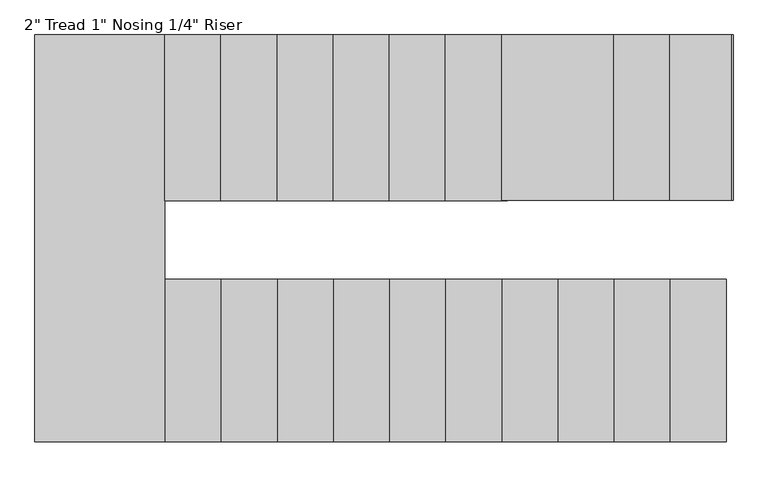
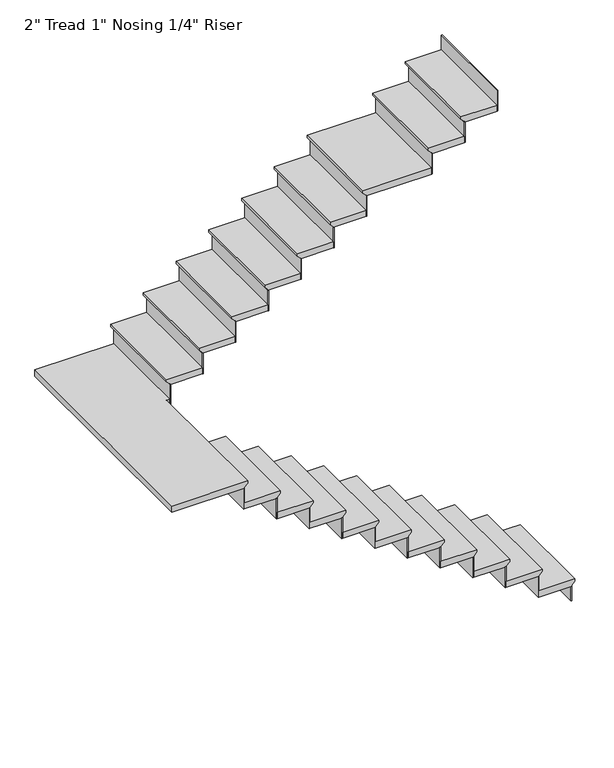
"""IFC4 building model written with IfcOpenShell, lengths in millimetres: stair flight geometry."""

from ifc_helpers import new_model, si_unit, origin, place, context, project, spatial, faceted_brep, source, transform, mapped, element, save


def stair_flight_05893867(model_context):
    return source(origin(), model_context, "Body", "Brep", [
        faceted_brep([(-3117.2664982, -7431.6600272, 150.2833333), (-3117.2664982, -7431.6600272, 169.3333333), (-3117.2664982, -8168.2600272, 169.3333333), (-3117.2664982, -8168.2600272, 150.2833333), (-3142.6664982, -7431.6600272, 124.8833333), (-3142.6664982, -8168.2600272, 124.8833333), (-3396.6664982, -7431.6600272, 169.3333333), (-3396.6664982, -8168.2600272, 169.3333333), (-3142.6664982, -8168.2600272, 118.5333333), (-3396.6664982, -8168.2600272, 118.5333333), (-3396.6664982, -7431.6600272, 118.5333333), (-3142.6664982, -7431.6600272, 118.5333333)], [[[0, 1, 2, 3]], [[4, 0, 3, 5]], [[2, 1, 6, 7]], [[8, 9, 10, 11]], [[2, 7, 9, 8, 5, 3]], [[8, 11, 4, 5]], [[6, 1, 0, 4, 11, 10]], [[7, 6, 10, 9]]]),
        faceted_brep([(-3142.6664982, -7431.6600272, 118.5333333), (-3142.6664982, -7431.6600272, 0.0), (-3149.0164982, -7431.6600272, 0.0), (-3149.0164982, -7431.6600272, 118.5333333), (-3142.6664982, -8168.2600272, 118.5333333), (-3149.0164982, -8168.2600272, 118.5333333), (-3149.0164982, -8168.2600272, 0.0), (-3142.6664982, -8168.2600272, 0.0)], [[[0, 1, 2, 3]], [[4, 5, 6, 7]], [[1, 0, 4, 7]], [[2, 1, 7, 6]], [[3, 2, 6, 5]], [[0, 3, 5, 4]]]),
        faceted_brep([(-3396.6664982, -7431.6600272, 287.8666667), (-3396.6664982, -7431.6600272, 118.5333333), (-3403.0164982, -7431.6600272, 118.5333333), (-3403.0164982, -7431.6600272, 287.8666667), (-3396.6664982, -8168.2600272, 287.8666667), (-3403.0164982, -8168.2600272, 287.8666667), (-3403.0164982, -8168.2600272, 118.5333333), (-3396.6664982, -8168.2600272, 118.5333333)], [[[0, 1, 2, 3]], [[4, 5, 6, 7]], [[1, 0, 4, 7]], [[2, 1, 7, 6]], [[3, 2, 6, 5]], [[0, 3, 5, 4]]]),
        faceted_brep([(-3371.2664982, -8168.2600272, 338.6666667), (-3371.2664982, -7431.6600272, 338.6666667), (-3650.6664982, -7431.6600272, 338.6666667), (-3650.6664982, -8168.2600272, 338.6666667), (-3396.6664982, -8168.2600272, 287.8666667), (-3650.6664982, -8168.2600272, 287.8666667), (-3650.6664982, -7431.6600272, 287.8666667), (-3396.6664982, -7431.6600272, 287.8666667), (-3396.6664982, -8168.2600272, 294.2166667), (-3371.2664982, -8168.2600272, 319.6166667), (-3396.6664982, -7431.6600272, 294.2166667), (-3371.2664982, -7431.6600272, 319.6166667)], [[[0, 1, 2, 3]], [[4, 5, 6, 7]], [[0, 3, 5, 4, 8, 9]], [[4, 7, 10, 8]], [[2, 1, 11, 10, 7, 6]], [[3, 2, 6, 5]], [[11, 1, 0, 9]], [[10, 11, 9, 8]]]),
        faceted_brep([(-3650.6664982, -7431.6600272, 457.2), (-3650.6664982, -7431.6600272, 287.8666667), (-3657.0164982, -7431.6600272, 287.8666667), (-3657.0164982, -7431.6600272, 457.2), (-3650.6664982, -8168.2600272, 457.2), (-3657.0164982, -8168.2600272, 457.2), (-3657.0164982, -8168.2600272, 287.8666667), (-3650.6664982, -8168.2600272, 287.8666667)], [[[0, 1, 2, 3]], [[4, 5, 6, 7]], [[1, 0, 4, 7]], [[2, 1, 7, 6]], [[3, 2, 6, 5]], [[0, 3, 5, 4]]]),
        faceted_brep([(-3625.2664982, -8168.2600272, 508.0), (-3625.2664982, -7431.6600272, 508.0), (-3904.6664982, -7431.6600272, 508.0), (-3904.6664982, -8168.2600272, 508.0), (-3650.6664982, -8168.2600272, 457.2), (-3904.6664982, -8168.2600272, 457.2), (-3904.6664982, -7431.6600272, 457.2), (-3650.6664982, -7431.6600272, 457.2), (-3650.6664982, -8168.2600272, 463.55), (-3625.2664982, -8168.2600272, 488.95), (-3650.6664982, -7431.6600272, 463.55), (-3625.2664982, -7431.6600272, 488.95)], [[[0, 1, 2, 3]], [[4, 5, 6, 7]], [[0, 3, 5, 4, 8, 9]], [[4, 7, 10, 8]], [[2, 1, 11, 10, 7, 6]], [[3, 2, 6, 5]], [[11, 1, 0, 9]], [[10, 11, 9, 8]]]),
        faceted_brep([(-3904.6664982, -7431.6600272, 626.5333333), (-3904.6664982, -7431.6600272, 457.2), (-3911.0164982, -7431.6600272, 457.2), (-3911.0164982, -7431.6600272, 626.5333333), (-3904.6664982, -8168.2600272, 626.5333333), (-3911.0164982, -8168.2600272, 626.5333333), (-3911.0164982, -8168.2600272, 457.2), (-3904.6664982, -8168.2600272, 457.2)], [[[0, 1, 2, 3]], [[4, 5, 6, 7]], [[1, 0, 4, 7]], [[2, 1, 7, 6]], [[3, 2, 6, 5]], [[0, 3, 5, 4]]]),
        faceted_brep([(-3879.2664982, -8168.2600272, 677.3333333), (-3879.2664982, -7431.6600272, 677.3333333), (-4158.6664982, -7431.6600272, 677.3333333), (-4158.6664982, -8168.2600272, 677.3333333), (-3904.6664982, -8168.2600272, 626.5333333), (-4158.6664982, -8168.2600272, 626.5333333), (-4158.6664982, -7431.6600272, 626.5333333), (-3904.6664982, -7431.6600272, 626.5333333), (-3904.6664982, -8168.2600272, 632.8833333), (-3879.2664982, -8168.2600272, 658.2833333), (-3904.6664982, -7431.6600272, 632.8833333), (-3879.2664982, -7431.6600272, 658.2833333)], [[[0, 1, 2, 3]], [[4, 5, 6, 7]], [[0, 3, 5, 4, 8, 9]], [[4, 7, 10, 8]], [[2, 1, 11, 10, 7, 6]], [[3, 2, 6, 5]], [[11, 1, 0, 9]], [[10, 11, 9, 8]]]),
        faceted_brep([(-4158.6664982, -7431.6600272, 795.8666667), (-4158.6664982, -7431.6600272, 626.5333333), (-4165.0164982, -7431.6600272, 626.5333333), (-4165.0164982, -7431.6600272, 795.8666667), (-4158.6664982, -8168.2600272, 795.8666667), (-4165.0164982, -8168.2600272, 795.8666667), (-4165.0164982, -8168.2600272, 626.5333333), (-4158.6664982, -8168.2600272, 626.5333333)], [[[0, 1, 2, 3]], [[4, 5, 6, 7]], [[1, 0, 4, 7]], [[2, 1, 7, 6]], [[3, 2, 6, 5]], [[0, 3, 5, 4]]]),
        faceted_brep([(-4133.2664982, -8168.2600272, 846.6666667), (-4133.2664982, -7431.6600272, 846.6666667), (-4412.6664982, -7431.6600272, 846.6666667), (-4412.6664982, -8168.2600272, 846.6666667), (-4158.6664982, -8168.2600272, 795.8666667), (-4412.6664982, -8168.2600272, 795.8666667), (-4412.6664982, -7431.6600272, 795.8666667), (-4158.6664982, -7431.6600272, 795.8666667), (-4158.6664982, -8168.2600272, 802.2166667), (-4133.2664982, -8168.2600272, 827.6166667), (-4158.6664982, -7431.6600272, 802.2166667), (-4133.2664982, -7431.6600272, 827.6166667)], [[[0, 1, 2, 3]], [[4, 5, 6, 7]], [[0, 3, 5, 4, 8, 9]], [[4, 7, 10, 8]], [[2, 1, 11, 10, 7, 6]], [[3, 2, 6, 5]], [[11, 1, 0, 9]], [[10, 11, 9, 8]]]),
        faceted_brep([(-4412.6664982, -7431.6600272, 965.2), (-4412.6664982, -7431.6600272, 795.8666667), (-4419.0164982, -7431.6600272, 795.8666667), (-4419.0164982, -7431.6600272, 965.2), (-4412.6664982, -8168.2600272, 965.2), (-4419.0164982, -8168.2600272, 965.2), (-4419.0164982, -8168.2600272, 795.8666667), (-4412.6664982, -8168.2600272, 795.8666667)], [[[0, 1, 2, 3]], [[4, 5, 6, 7]], [[1, 0, 4, 7]], [[2, 1, 7, 6]], [[3, 2, 6, 5]], [[0, 3, 5, 4]]]),
        faceted_brep([(-4387.2664982, -8168.2600272, 1016.0), (-4387.2664982, -7431.6600272, 1016.0), (-4666.6664982, -7431.6600272, 1016.0), (-4666.6664982, -8168.2600272, 1016.0), (-4412.6664982, -8168.2600272, 965.2), (-4666.6664982, -8168.2600272, 965.2), (-4666.6664982, -7431.6600272, 965.2), (-4412.6664982, -7431.6600272, 965.2), (-4412.6664982, -8168.2600272, 971.55), (-4387.2664982, -8168.2600272, 996.95), (-4412.6664982, -7431.6600272, 971.55), (-4387.2664982, -7431.6600272, 996.95)], [[[0, 1, 2, 3]], [[4, 5, 6, 7]], [[0, 3, 5, 4, 8, 9]], [[4, 7, 10, 8]], [[2, 1, 11, 10, 7, 6]], [[3, 2, 6, 5]], [[11, 1, 0, 9]], [[10, 11, 9, 8]]]),
        faceted_brep([(-4666.6664982, -7431.6600272, 1134.5333333), (-4666.6664982, -7431.6600272, 965.2), (-4673.0164982, -7431.6600272, 965.2), (-4673.0164982, -7431.6600272, 1134.5333333), (-4666.6664982, -8168.2600272, 1134.5333333), (-4673.0164982, -8168.2600272, 1134.5333333), (-4673.0164982, -8168.2600272, 965.2), (-4666.6664982, -8168.2600272, 965.2)], [[[0, 1, 2, 3]], [[4, 5, 6, 7]], [[1, 0, 4, 7]], [[2, 1, 7, 6]], [[3, 2, 6, 5]], [[0, 3, 5, 4]]]),
        faceted_brep([(-4641.2664982, -8168.2600272, 1185.3333333), (-4641.2664982, -7431.6600272, 1185.3333333), (-4920.6664982, -7431.6600272, 1185.3333333), (-4920.6664982, -8168.2600272, 1185.3333333), (-4666.6664982, -8168.2600272, 1134.5333333), (-4920.6664982, -8168.2600272, 1134.5333333), (-4920.6664982, -7431.6600272, 1134.5333333), (-4666.6664982, -7431.6600272, 1134.5333333), (-4666.6664982, -8168.2600272, 1140.8833333), (-4641.2664982, -8168.2600272, 1166.2833333), (-4666.6664982, -7431.6600272, 1140.8833333), (-4641.2664982, -7431.6600272, 1166.2833333)], [[[0, 1, 2, 3]], [[4, 5, 6, 7]], [[0, 3, 5, 4, 8, 9]], [[4, 7, 10, 8]], [[2, 1, 11, 10, 7, 6]], [[3, 2, 6, 5]], [[11, 1, 0, 9]], [[10, 11, 9, 8]]]),
        faceted_brep([(-4920.6664982, -7431.6600272, 1303.8666667), (-4920.6664982, -7431.6600272, 1134.5333333), (-4927.0164982, -7431.6600272, 1134.5333333), (-4927.0164982, -7431.6600272, 1303.8666667), (-4920.6664982, -8168.2600272, 1303.8666667), (-4927.0164982, -8168.2600272, 1303.8666667), (-4927.0164982, -8168.2600272, 1134.5333333), (-4920.6664982, -8168.2600272, 1134.5333333)], [[[0, 1, 2, 3]], [[4, 5, 6, 7]], [[1, 0, 4, 7]], [[2, 1, 7, 6]], [[3, 2, 6, 5]], [[0, 3, 5, 4]]]),
        faceted_brep([(-4895.2664982, -8168.2600272, 1354.6666667), (-4895.2664982, -7431.6600272, 1354.6666667), (-5174.6664982, -7431.6600272, 1354.6666667), (-5174.6664982, -8168.2600272, 1354.6666667), (-4920.6664982, -8168.2600272, 1303.8666667), (-5174.6664982, -8168.2600272, 1303.8666667), (-5174.6664982, -7431.6600272, 1303.8666667), (-4920.6664982, -7431.6600272, 1303.8666667), (-4920.6664982, -8168.2600272, 1310.2166667), (-4895.2664982, -8168.2600272, 1335.6166667), (-4920.6664982, -7431.6600272, 1310.2166667), (-4895.2664982, -7431.6600272, 1335.6166667)], [[[0, 1, 2, 3]], [[4, 5, 6, 7]], [[0, 3, 5, 4, 8, 9]], [[4, 7, 10, 8]], [[2, 1, 11, 10, 7, 6]], [[3, 2, 6, 5]], [[11, 1, 0, 9]], [[10, 11, 9, 8]]]),
        faceted_brep([(-5174.6664982, -7431.6600272, 1473.2), (-5174.6664982, -7431.6600272, 1303.8666667), (-5181.0164982, -7431.6600272, 1303.8666667), (-5181.0164982, -7431.6600272, 1473.2), (-5174.6664982, -8168.2600272, 1473.2), (-5181.0164982, -8168.2600272, 1473.2), (-5181.0164982, -8168.2600272, 1303.8666667), (-5174.6664982, -8168.2600272, 1303.8666667)], [[[0, 1, 2, 3]], [[4, 5, 6, 7]], [[1, 0, 4, 7]], [[2, 1, 7, 6]], [[3, 2, 6, 5]], [[0, 3, 5, 4]]]),
        faceted_brep([(-5149.2664982, -8168.2600272, 1524.0), (-5149.2664982, -7431.6600272, 1524.0), (-5428.6664982, -7431.6600272, 1524.0), (-5428.6664982, -8168.2600272, 1524.0), (-5174.6664982, -8168.2600272, 1473.2), (-5428.6664982, -8168.2600272, 1473.2), (-5428.6664982, -7431.6600272, 1473.2), (-5174.6664982, -7431.6600272, 1473.2), (-5174.6664982, -8168.2600272, 1479.55), (-5149.2664982, -8168.2600272, 1504.95), (-5174.6664982, -7431.6600272, 1479.55), (-5149.2664982, -7431.6600272, 1504.95)], [[[0, 1, 2, 3]], [[4, 5, 6, 7]], [[0, 3, 5, 4, 8, 9]], [[4, 7, 10, 8]], [[2, 1, 11, 10, 7, 6]], [[3, 2, 6, 5]], [[11, 1, 0, 9]], [[10, 11, 9, 8]]]),
        faceted_brep([(-5428.6664982, -7431.6600272, 1642.5333333), (-5428.6664982, -7431.6600272, 1473.2), (-5435.0164982, -7431.6600272, 1473.2), (-5435.0164982, -7431.6600272, 1642.5333333), (-5428.6664982, -8168.2600272, 1642.5333333), (-5435.0164982, -8168.2600272, 1642.5333333), (-5435.0164982, -8168.2600272, 1473.2), (-5428.6664982, -8168.2600272, 1473.2)], [[[0, 1, 2, 3]], [[4, 5, 6, 7]], [[1, 0, 4, 7]], [[2, 1, 7, 6]], [[3, 2, 6, 5]], [[0, 3, 5, 4]]]),
        faceted_brep([(-5403.2664982, -8168.2600272, 1693.3333333), (-5403.2664982, -7431.6600272, 1693.3333333), (-5682.6664982, -7431.6600272, 1693.3333333), (-5682.6664982, -8168.2600272, 1693.3333333), (-5428.6664982, -8168.2600272, 1642.5333333), (-5682.6664982, -8168.2600272, 1642.5333333), (-5682.6664982, -7431.6600272, 1642.5333333), (-5428.6664982, -7431.6600272, 1642.5333333), (-5428.6664982, -8168.2600272, 1648.8833333), (-5403.2664982, -8168.2600272, 1674.2833333), (-5428.6664982, -7431.6600272, 1648.8833333), (-5403.2664982, -7431.6600272, 1674.2833333)], [[[0, 1, 2, 3]], [[4, 5, 6, 7]], [[0, 3, 5, 4, 8, 9]], [[4, 7, 10, 8]], [[2, 1, 11, 10, 7, 6]], [[3, 2, 6, 5]], [[11, 1, 0, 9]], [[10, 11, 9, 8]]]),
        faceted_brep([(-5682.6664982, -7431.6600272, 1811.8666667), (-5682.6664982, -7431.6600272, 1642.5333333), (-5689.0164982, -7431.6600272, 1642.5333333), (-5689.0164982, -7431.6600272, 1811.8666667), (-5682.6664982, -8168.2600272, 1811.8666667), (-5689.0164982, -8168.2600272, 1811.8666667), (-5689.0164982, -8168.2600272, 1642.5333333), (-5682.6664982, -8168.2600272, 1642.5333333)], [[[0, 1, 2, 3]], [[4, 5, 6, 7]], [[1, 0, 4, 7]], [[2, 1, 7, 6]], [[3, 2, 6, 5]], [[0, 3, 5, 4]]]),
        faceted_brep([(-5631.8664982, -6326.7600272, 1862.6666667), (-6245.2108866, -6326.7600272, 1862.6666667), (-6245.2108866, -8168.2600272, 1862.6666667), (-5657.2664982, -8168.2600272, 1862.6666667), (-5657.2664982, -7076.0600272, 1862.6666667), (-5631.8664982, -7076.0600272, 1862.6666667), (-6245.2108866, -6326.7600272, 1811.8666667), (-5631.8664982, -6326.7600272, 1811.8666667), (-5631.8664982, -7076.0600272, 1811.8666667), (-5657.2664982, -7076.0600272, 1811.8666667), (-5657.2664982, -7431.6600272, 1811.8666667), (-5682.6664982, -7431.6600272, 1811.8666667), (-5682.6664982, -8168.2600272, 1811.8666667), (-6245.2108866, -8168.2600272, 1811.8666667), (-5682.6664982, -8168.2600272, 1818.2166667), (-5657.2664982, -8168.2600272, 1843.6166667), (-5682.6664982, -7431.6600272, 1818.2166667), (-5657.2664982, -7431.6600272, 1843.6166667)], [[[0, 1, 2, 3, 4, 5]], [[6, 7, 8, 9, 10, 11, 12, 13]], [[1, 0, 7, 6]], [[2, 1, 6, 13]], [[3, 2, 13, 12, 14, 15]], [[12, 11, 16, 14]], [[11, 10, 17, 16]], [[4, 3, 15, 17, 10, 9]], [[5, 4, 9, 8]], [[0, 5, 8, 7]], [[15, 14, 16, 17]]]),
        faceted_brep([(-5631.8664982, -7076.0600272, 1981.2), (-5631.8664982, -7076.0600272, 1811.8666667), (-5625.5164982, -7076.0600272, 1811.8666667), (-5625.5164982, -7076.0600272, 1981.2), (-5631.8664982, -6326.7600272, 1981.2), (-5625.5164982, -6326.7600272, 1981.2), (-5625.5164982, -6326.7600272, 1811.8666667), (-5631.8664982, -6326.7600272, 1811.8666667)], [[[0, 1, 2, 3]], [[4, 5, 6, 7]], [[1, 0, 4, 7]], [[2, 1, 7, 6]], [[3, 2, 6, 5]], [[0, 3, 5, 4]]]),
        faceted_brep([(-5657.2664982, -6326.7600272, 2032.0), (-5657.2664982, -7076.0600272, 2032.0), (-5377.8664982, -7076.0600272, 2032.0), (-5377.8664982, -6326.7600272, 2032.0), (-5631.8664982, -6326.7600272, 1981.2), (-5377.8664982, -6326.7600272, 1981.2), (-5377.8664982, -7076.0600272, 1981.2), (-5631.8664982, -7076.0600272, 1981.2), (-5631.8664982, -6326.7600272, 1987.55), (-5657.2664982, -6326.7600272, 2012.95), (-5631.8664982, -7076.0600272, 1987.55), (-5657.2664982, -7076.0600272, 2012.95)], [[[0, 1, 2, 3]], [[4, 5, 6, 7]], [[0, 3, 5, 4, 8, 9]], [[4, 7, 10, 8]], [[2, 1, 11, 10, 7, 6]], [[3, 2, 6, 5]], [[11, 1, 0, 9]], [[10, 11, 9, 8]]]),
        faceted_brep([(-5377.8664982, -7076.0600272, 2150.5333333), (-5377.8664982, -7076.0600272, 1981.2), (-5371.5164982, -7076.0600272, 1981.2), (-5371.5164982, -7076.0600272, 2150.5333333), (-5377.8664982, -6326.7600272, 2150.5333333), (-5371.5164982, -6326.7600272, 2150.5333333), (-5371.5164982, -6326.7600272, 1981.2), (-5377.8664982, -6326.7600272, 1981.2)], [[[0, 1, 2, 3]], [[4, 5, 6, 7]], [[1, 0, 4, 7]], [[2, 1, 7, 6]], [[3, 2, 6, 5]], [[0, 3, 5, 4]]]),
        faceted_brep([(-5403.2664982, -6326.7600272, 2201.3333333), (-5403.2664982, -7076.0600272, 2201.3333333), (-5123.8664982, -7076.0600272, 2201.3333333), (-5123.8664982, -6326.7600272, 2201.3333333), (-5377.8664982, -6326.7600272, 2150.5333333), (-5123.8664982, -6326.7600272, 2150.5333333), (-5123.8664982, -7076.0600272, 2150.5333333), (-5377.8664982, -7076.0600272, 2150.5333333), (-5377.8664982, -6326.7600272, 2156.8833333), (-5403.2664982, -6326.7600272, 2182.2833333), (-5377.8664982, -7076.0600272, 2156.8833333), (-5403.2664982, -7076.0600272, 2182.2833333)], [[[0, 1, 2, 3]], [[4, 5, 6, 7]], [[0, 3, 5, 4, 8, 9]], [[4, 7, 10, 8]], [[2, 1, 11, 10, 7, 6]], [[3, 2, 6, 5]], [[11, 1, 0, 9]], [[10, 11, 9, 8]]]),
        faceted_brep([(-5123.8664982, -7076.0600272, 2319.8666667), (-5123.8664982, -7076.0600272, 2150.5333333), (-5117.5164982, -7076.0600272, 2150.5333333), (-5117.5164982, -7076.0600272, 2319.8666667), (-5123.8664982, -6326.7600272, 2319.8666667), (-5117.5164982, -6326.7600272, 2319.8666667), (-5117.5164982, -6326.7600272, 2150.5333333), (-5123.8664982, -6326.7600272, 2150.5333333)], [[[0, 1, 2, 3]], [[4, 5, 6, 7]], [[1, 0, 4, 7]], [[2, 1, 7, 6]], [[3, 2, 6, 5]], [[0, 3, 5, 4]]]),
        faceted_brep([(-5149.2664982, -6326.7600272, 2370.6666667), (-5149.2664982, -7076.0600272, 2370.6666667), (-4869.8664982, -7076.0600272, 2370.6666667), (-4869.8664982, -6326.7600272, 2370.6666667), (-5123.8664982, -6326.7600272, 2319.8666667), (-4869.8664982, -6326.7600272, 2319.8666667), (-4869.8664982, -7076.0600272, 2319.8666667), (-5123.8664982, -7076.0600272, 2319.8666667), (-5123.8664982, -6326.7600272, 2326.2166667), (-5149.2664982, -6326.7600272, 2351.6166667), (-5123.8664982, -7076.0600272, 2326.2166667), (-5149.2664982, -7076.0600272, 2351.6166667)], [[[0, 1, 2, 3]], [[4, 5, 6, 7]], [[0, 3, 5, 4, 8, 9]], [[4, 7, 10, 8]], [[2, 1, 11, 10, 7, 6]], [[3, 2, 6, 5]], [[11, 1, 0, 9]], [[10, 11, 9, 8]]]),
        faceted_brep([(-4869.8664982, -7076.0600272, 2489.2), (-4869.8664982, -7076.0600272, 2319.8666667), (-4863.5164982, -7076.0600272, 2319.8666667), (-4863.5164982, -7076.0600272, 2489.2), (-4869.8664982, -6326.7600272, 2489.2), (-4863.5164982, -6326.7600272, 2489.2), (-4863.5164982, -6326.7600272, 2319.8666667), (-4869.8664982, -6326.7600272, 2319.8666667)], [[[0, 1, 2, 3]], [[4, 5, 6, 7]], [[1, 0, 4, 7]], [[2, 1, 7, 6]], [[3, 2, 6, 5]], [[0, 3, 5, 4]]]),
        faceted_brep([(-4895.2664982, -6326.7600272, 2540.0), (-4895.2664982, -7076.0600272, 2540.0), (-4615.8664982, -7076.0600272, 2540.0), (-4615.8664982, -6326.7600272, 2540.0), (-4869.8664982, -6326.7600272, 2489.2), (-4615.8664982, -6326.7600272, 2489.2), (-4615.8664982, -7076.0600272, 2489.2), (-4869.8664982, -7076.0600272, 2489.2), (-4869.8664982, -6326.7600272, 2495.55), (-4895.2664982, -6326.7600272, 2520.95), (-4869.8664982, -7076.0600272, 2495.55), (-4895.2664982, -7076.0600272, 2520.95)], [[[0, 1, 2, 3]], [[4, 5, 6, 7]], [[0, 3, 5, 4, 8, 9]], [[4, 7, 10, 8]], [[2, 1, 11, 10, 7, 6]], [[3, 2, 6, 5]], [[11, 1, 0, 9]], [[10, 11, 9, 8]]]),
        faceted_brep([(-4615.8664982, -7076.0600272, 2658.5333333), (-4615.8664982, -7076.0600272, 2489.2), (-4609.5164982, -7076.0600272, 2489.2), (-4609.5164982, -7076.0600272, 2658.5333333), (-4615.8664982, -6326.7600272, 2658.5333333), (-4609.5164982, -6326.7600272, 2658.5333333), (-4609.5164982, -6326.7600272, 2489.2), (-4615.8664982, -6326.7600272, 2489.2)], [[[0, 1, 2, 3]], [[4, 5, 6, 7]], [[1, 0, 4, 7]], [[2, 1, 7, 6]], [[3, 2, 6, 5]], [[0, 3, 5, 4]]]),
        faceted_brep([(-4641.2664982, -6326.7600272, 2709.3333333), (-4641.2664982, -7076.0600272, 2709.3333333), (-4361.8664982, -7076.0600272, 2709.3333333), (-4361.8664982, -6326.7600272, 2709.3333333), (-4615.8664982, -6326.7600272, 2658.5333333), (-4361.8664982, -6326.7600272, 2658.5333333), (-4361.8664982, -7076.0600272, 2658.5333333), (-4615.8664982, -7076.0600272, 2658.5333333), (-4615.8664982, -6326.7600272, 2664.8833333), (-4641.2664982, -6326.7600272, 2690.2833333), (-4615.8664982, -7076.0600272, 2664.8833333), (-4641.2664982, -7076.0600272, 2690.2833333)], [[[0, 1, 2, 3]], [[4, 5, 6, 7]], [[0, 3, 5, 4, 8, 9]], [[4, 7, 10, 8]], [[2, 1, 11, 10, 7, 6]], [[3, 2, 6, 5]], [[11, 1, 0, 9]], [[10, 11, 9, 8]]]),
        faceted_brep([(-4361.8664982, -7076.0600272, 2827.8666667), (-4361.8664982, -7076.0600272, 2658.5333333), (-4355.5164982, -7076.0600272, 2658.5333333), (-4355.5164982, -7076.0600272, 2827.8666667), (-4361.8664982, -6326.7600272, 2827.8666667), (-4355.5164982, -6326.7600272, 2827.8666667), (-4355.5164982, -6326.7600272, 2658.5333333), (-4361.8664982, -6326.7600272, 2658.5333333)], [[[0, 1, 2, 3]], [[4, 5, 6, 7]], [[1, 0, 4, 7]], [[2, 1, 7, 6]], [[3, 2, 6, 5]], [[0, 3, 5, 4]]]),
        faceted_brep([(-4387.2664982, -6326.7600272, 2878.6666667), (-4387.2664982, -7076.0600272, 2878.6666667), (-4107.8664982, -7076.0600272, 2878.6666667), (-4107.8664982, -6326.7600272, 2878.6666667), (-4361.8664982, -6326.7600272, 2827.8666667), (-4107.8664982, -6326.7600272, 2827.8666667), (-4107.8664982, -7076.0600272, 2827.8666667), (-4361.8664982, -7076.0600272, 2827.8666667), (-4361.8664982, -6326.7600272, 2834.2166667), (-4387.2664982, -6326.7600272, 2859.6166667), (-4361.8664982, -7076.0600272, 2834.2166667), (-4387.2664982, -7076.0600272, 2859.6166667)], [[[0, 1, 2, 3]], [[4, 5, 6, 7]], [[0, 3, 5, 4, 8, 9]], [[4, 7, 10, 8]], [[2, 1, 11, 10, 7, 6]], [[3, 2, 6, 5]], [[11, 1, 0, 9]], [[10, 11, 9, 8]]]),
        faceted_brep([(-4107.8664982, -7076.0600272, 2997.2), (-4107.8664982, -7076.0600272, 2827.8666667), (-4101.5164982, -7076.0600272, 2827.8666667), (-4101.5164982, -7076.0600272, 2997.2), (-4107.8664982, -6326.7600272, 2997.2), (-4101.5164982, -6326.7600272, 2997.2), (-4101.5164982, -6326.7600272, 2827.8666667), (-4107.8664982, -6326.7600272, 2827.8666667)], [[[0, 1, 2, 3]], [[4, 5, 6, 7]], [[1, 0, 4, 7]], [[2, 1, 7, 6]], [[3, 2, 6, 5]], [[0, 3, 5, 4]]]),
        faceted_brep([(-4133.2664982, -6326.7600272, 3048.0), (-4133.2664982, -7076.0600272, 3048.0), (-3599.8664982, -7076.0600272, 3048.0), (-3599.8664982, -6326.7600272, 3048.0), (-4107.8664982, -6326.7600272, 2997.2), (-3599.8664982, -6326.7600272, 2997.2), (-3599.8664982, -7076.0600272, 2997.2), (-4107.8664982, -7076.0600272, 2997.2), (-4107.8664982, -6326.7600272, 3003.55), (-4133.2664982, -6326.7600272, 3028.95), (-4107.8664982, -7076.0600272, 3003.55), (-4133.2664982, -7076.0600272, 3028.95)], [[[0, 1, 2, 3]], [[4, 5, 6, 7]], [[0, 3, 5, 4, 8, 9]], [[4, 7, 10, 8]], [[2, 1, 11, 10, 7, 6]], [[3, 2, 6, 5]], [[11, 1, 0, 9]], [[10, 11, 9, 8]]]),
        faceted_brep([(-3599.8664982, -7076.0600272, 3166.5333333), (-3599.8664982, -7076.0600272, 2997.2), (-3593.5164982, -7076.0600272, 2997.2), (-3593.5164982, -7076.0600272, 3166.5333333), (-3599.8664982, -6326.7600272, 3166.5333333), (-3593.5164982, -6326.7600272, 3166.5333333), (-3593.5164982, -6326.7600272, 2997.2), (-3599.8664982, -6326.7600272, 2997.2)], [[[0, 1, 2, 3]], [[4, 5, 6, 7]], [[1, 0, 4, 7]], [[2, 1, 7, 6]], [[3, 2, 6, 5]], [[0, 3, 5, 4]]]),
        faceted_brep([(-3625.2664982, -6326.7600272, 3217.3333333), (-3625.2664982, -7076.0600272, 3217.3333333), (-3345.8664982, -7076.0600272, 3217.3333333), (-3345.8664982, -6326.7600272, 3217.3333333), (-3599.8664982, -6326.7600272, 3166.5333333), (-3345.8664982, -6326.7600272, 3166.5333333), (-3345.8664982, -7076.0600272, 3166.5333333), (-3599.8664982, -7076.0600272, 3166.5333333), (-3599.8664982, -6326.7600272, 3172.8833333), (-3625.2664982, -6326.7600272, 3198.2833333), (-3599.8664982, -7076.0600272, 3172.8833333), (-3625.2664982, -7076.0600272, 3198.2833333)], [[[0, 1, 2, 3]], [[4, 5, 6, 7]], [[0, 3, 5, 4, 8, 9]], [[4, 7, 10, 8]], [[2, 1, 11, 10, 7, 6]], [[3, 2, 6, 5]], [[11, 1, 0, 9]], [[10, 11, 9, 8]]]),
        faceted_brep([(-3345.8664982, -7076.0600272, 3335.8666667), (-3345.8664982, -7076.0600272, 3166.5333333), (-3339.5164982, -7076.0600272, 3166.5333333), (-3339.5164982, -7076.0600272, 3335.8666667), (-3345.8664982, -6326.7600272, 3335.8666667), (-3339.5164982, -6326.7600272, 3335.8666667), (-3339.5164982, -6326.7600272, 3166.5333333), (-3345.8664982, -6326.7600272, 3166.5333333)], [[[0, 1, 2, 3]], [[4, 5, 6, 7]], [[1, 0, 4, 7]], [[2, 1, 7, 6]], [[3, 2, 6, 5]], [[0, 3, 5, 4]]]),
        faceted_brep([(-3091.8664982, -7076.0600272, 3505.2), (-3091.8664982, -7076.0600272, 3335.8666667), (-3085.5164982, -7076.0600272, 3335.8666667), (-3085.5164982, -7076.0600272, 3505.2), (-3091.8664982, -6326.7600272, 3505.2), (-3085.5164982, -6326.7600272, 3505.2), (-3085.5164982, -6326.7600272, 3335.8666667), (-3091.8664982, -6326.7600272, 3335.8666667)], [[[0, 1, 2, 3]], [[4, 5, 6, 7]], [[1, 0, 4, 7]], [[2, 1, 7, 6]], [[3, 2, 6, 5]], [[0, 3, 5, 4]]]),
        faceted_brep([(-3371.2664982, -6326.7600272, 3386.6666667), (-3371.2664982, -7076.0600272, 3386.6666667), (-3091.8664982, -7076.0600272, 3386.6666667), (-3091.8664982, -6326.7600272, 3386.6666667), (-3345.8664982, -6326.7600272, 3335.8666667), (-3091.8664982, -6326.7600272, 3335.8666667), (-3091.8664982, -7076.0600272, 3335.8666667), (-3345.8664982, -7076.0600272, 3335.8666667), (-3345.8664982, -6326.7600272, 3342.2166667), (-3371.2664982, -6326.7600272, 3367.6166667), (-3345.8664982, -7076.0600272, 3342.2166667), (-3371.2664982, -7076.0600272, 3367.6166667)], [[[0, 1, 2, 3]], [[4, 5, 6, 7]], [[0, 3, 5, 4, 8, 9]], [[4, 7, 10, 8]], [[2, 1, 11, 10, 7, 6]], [[3, 2, 6, 5]], [[11, 1, 0, 9]], [[10, 11, 9, 8]]]),
    ])


if __name__ == "__main__":
    model = new_model("IFC4")
    model_context = context("Model", 3, world=origin())
    ifc_project = project(units=[si_unit("LENGTHUNIT", "METRE", prefix="MILLI")], contexts=[model_context])
    site = spatial("IfcSite", under=ifc_project)
    building = spatial("IfcBuilding", under=site)
    placement = place(None, origin())
    stair_flight_shape = stair_flight_05893867(model_context)
    element("IfcStairFlight", 1, ObjectType="2\" Tread 1\" Nosing 1/4\" Riser", at=placement, inside=building, context=model_context, shape_type="MappedRepresentation", body=[
        mapped(stair_flight_shape, transform((0.0, 0.0, 0.0), x_axis=(1.0, 0.0, 0.0), y_axis=(0.0, 1.0, 0.0), z_axis=(0.0, 0.0, 1.0))),
    ])
    save(model, "model.ifc")
